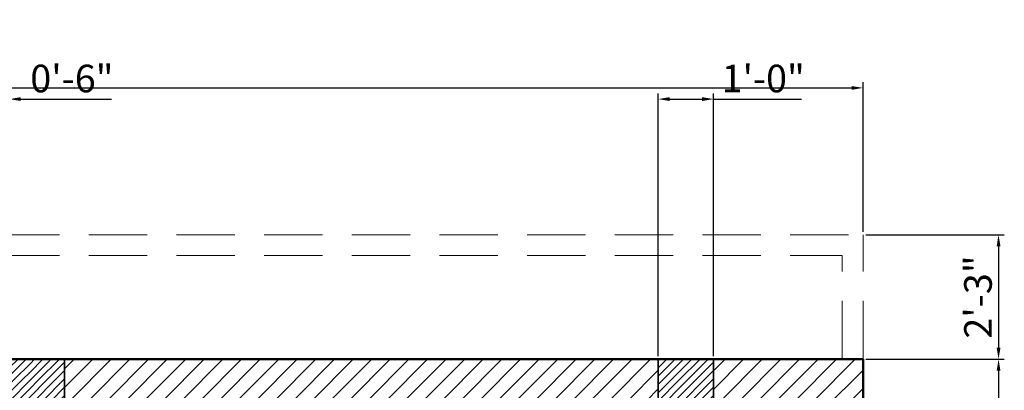
# Model space of a CAD drawing. Units: millimetres. Extents: x 225995 to 227247, y 225507 to 226008.
# Tile 23 of 23: x 227029 to 227243, y 225928 to 226008. Entities that reach past the tile are written whole.
import ezdxf

# ---------------------------------------------------------------- set-up
doc = ezdxf.new("R2010")
doc.units = ezdxf.units.MM
doc.linetypes.add('DASHED', pattern=[19.05, 12.7, -6.35])
for name, color, linetype, lineweight in [('A-ANNO-DIMS', 2, 'Continuous', 18), ('A-COLS', 40, 'Continuous', 35), ('A-WALL', 7, 'Continuous', 50), ('A-WALL-OVHD', 1, 'DASHED', 18), ('A-WALL-PATT', 8, 'Continuous', 13)]:
    doc.layers.add(name, color=color, linetype=linetype, lineweight=lineweight)
doc.styles.get("Standard").update_dxf_attribs({"font": 'arial.ttf'})
doc.dimstyles.new('ISO-25', dxfattribs={"dimtxt": 6, "dimasz": 2.5, "dimexe": 1.25, "dimexo": 0.625, "dimtad": 1, "dimdec": 0, "dimlunit": 3, "dimtxsty": 'Standard', "dimcen": 2.5, "dimadec": 0, "dimazin": 0, "dimtfac": 1, "dimtdec": 0, "dimtmove": 0, "dimatfit": 3, "dimfxl": 1, "dimarcsym": 0})
pattern_1 = [(45, (646.0463, 0.931), (-2.020557627, 2.020557627), [])]
pattern_2 = [(45, (787.0463, 234.931), (-0.898025612, 0.898025612), [])]
pattern_3 = [(45, (646.0463, 234.931), (-0.898025612, 0.898025612), [])]

# ---------------------------------------------------------------- blocks, each defined once
blk = doc.blocks.new('*D70')
at = {"layer": 'A-ANNO-DIMS', "color": 0, "lineweight": -2, "transparency": 16777216}
for p, q in [((226679.92, 225962.33), (226679.92, 225994.83)), ((226682.42, 225993.58), (227209.42, 225993.58)), ((227211.92, 225962.33), (227211.92, 225994.83))]:
    blk.add_line(p, q, dxfattribs=at)
at = {"layer": 'A-ANNO-DIMS', "color": 0, "transparency": 16777216}
for points in [[(226682.42, 225993.99), (226682.42, 225993.16), (226679.92, 225993.58)], [(227209.42, 225993.99), (227209.42, 225993.16), (227211.92, 225993.58)]]:
    blk.add_solid(points, dxfattribs=at)
at = {"layer": 'Defpoints', "color": 0, "transparency": 16777216}
for p in [(227211.92, 225993.58), (226679.92, 225961.7), (227211.92, 225961.7)]:
    blk.add_point(p, dxfattribs=at)
at = {"layer": 'A-ANNO-DIMS', "color": 0, "transparency": 16777216, "insert": (226945.92, 226000.2), "char_height": 12, "attachment_point": 5}
blk.add_mtext('44\'-4"', dxfattribs=at)
blk = doc.blocks.new('*D121')
at = {"layer": 'A-ANNO-DIMS', "color": 0, "lineweight": -2, "transparency": 16777216}
for p, q in [((227017.92, 225991.15), (227015.42, 225991.15)), ((227020.42, 225935.33), (227020.42, 225992.4)), ((227020.42, 225991.15), (227026.42, 225991.15)), ((227026.42, 225935.33), (227026.42, 225992.4)), ((227028.92, 225991.15), (227048.62, 225991.15))]:
    blk.add_line(p, q, dxfattribs=at)
at = {"layer": 'A-ANNO-DIMS', "color": 0, "transparency": 16777216}
for points in [[(227017.92, 225991.57), (227017.92, 225990.74), (227020.42, 225991.15)], [(227028.92, 225991.57), (227028.92, 225990.74), (227026.42, 225991.15)]]:
    blk.add_solid(points, dxfattribs=at)
at = {"layer": 'Defpoints', "color": 0, "transparency": 16777216}
for p in [(227026.42, 225991.15), (227020.42, 225934.7), (227026.42, 225934.7)]:
    blk.add_point(p, dxfattribs=at)
at = {"layer": 'A-ANNO-DIMS', "color": 0, "transparency": 16777216, "insert": (227040.02, 225994.84), "char_height": 6, "attachment_point": 5}
blk.add_mtext('0\'-6"', dxfattribs=at)
blk = doc.blocks.new('*D122')
at = {"layer": 'A-ANNO-DIMS', "color": 0, "lineweight": -2, "transparency": 16777216}
for p, q in [((227167.42, 225935.33), (227167.42, 225992.4)), ((227169.92, 225991.15), (227176.92, 225991.15)), ((227179.42, 225935.33), (227179.42, 225992.4)), ((227179.42, 225991.15), (227198.56, 225991.15))]:
    blk.add_line(p, q, dxfattribs=at)
at = {"layer": 'A-ANNO-DIMS', "color": 0, "transparency": 16777216}
for points in [[(227169.92, 225991.57), (227169.92, 225990.74), (227167.42, 225991.15)], [(227176.92, 225991.57), (227176.92, 225990.74), (227179.42, 225991.15)]]:
    blk.add_solid(points, dxfattribs=at)
at = {"layer": 'Defpoints', "color": 0, "transparency": 16777216}
for p in [(227179.42, 225991.15), (227167.42, 225934.7), (227179.42, 225934.7)]:
    blk.add_point(p, dxfattribs=at)
at = {"layer": 'A-ANNO-DIMS', "color": 0, "transparency": 16777216, "insert": (227190.24, 225994.84), "char_height": 6, "attachment_point": 5}
blk.add_mtext('1\'-0"', dxfattribs=at)
blk = doc.blocks.new('*D123')
at = {"layer": 'A-ANNO-DIMS', "color": 0, "lineweight": -2, "transparency": 16777216}
for p, q in [((227212.55, 225961.7), (227242.62, 225961.7)), ((227241.37, 225959.2), (227241.37, 225937.2)), ((227212.55, 225934.7), (227242.62, 225934.7))]:
    blk.add_line(p, q, dxfattribs=at)
at = {"layer": 'A-ANNO-DIMS', "color": 0, "transparency": 16777216}
for points in [[(227240.96, 225959.2), (227241.79, 225959.2), (227241.37, 225961.7)], [(227240.96, 225937.2), (227241.79, 225937.2), (227241.37, 225934.7)]]:
    blk.add_solid(points, dxfattribs=at)
at = {"layer": 'Defpoints', "color": 0, "transparency": 16777216}
for p in [(227211.92, 225961.7), (227211.92, 225934.7), (227241.37, 225934.7)]:
    blk.add_point(p, dxfattribs=at)
at = {"layer": 'A-ANNO-DIMS', "color": 0, "transparency": 16777216, "insert": (227237.68, 225948.2), "char_height": 6, "attachment_point": 5, "rotation": 90}
blk.add_mtext('2\'-3"', dxfattribs=at)
blk = doc.blocks.new('*D124')
at = {"layer": 'A-ANNO-DIMS', "color": 0, "lineweight": -2, "transparency": 16777216}
for p, q in [((227212.55, 225934.7), (227242.62, 225934.7)), ((227241.37, 225932.2), (227241.37, 225880.2)), ((227212.55, 225877.7), (227242.62, 225877.7))]:
    blk.add_line(p, q, dxfattribs=at)
at = {"layer": 'A-ANNO-DIMS', "color": 0, "transparency": 16777216}
for points in [[(227240.96, 225932.2), (227241.79, 225932.2), (227241.37, 225934.7)], [(227240.96, 225880.2), (227241.79, 225880.2), (227241.37, 225877.7)]]:
    blk.add_solid(points, dxfattribs=at)
at = {"layer": 'Defpoints', "color": 0, "transparency": 16777216}
for p in [(227211.92, 225934.7), (227211.92, 225877.7), (227241.37, 225877.7)]:
    blk.add_point(p, dxfattribs=at)
at = {"layer": 'A-ANNO-DIMS', "color": 0, "transparency": 16777216, "insert": (227237.68, 225906.2), "char_height": 6, "attachment_point": 5, "rotation": 90}
blk.add_mtext('4\'-9"', dxfattribs=at)

msp = doc.modelspace()

# ---------------------------------------------------------------- hatches: boundary and pattern name
at = {"layer": 'A-WALL-PATT'}
h = msp.add_hatch(dxfattribs=at)
h.set_pattern_fill('ANSI31', color=256, scale=0.4)
h.set_pattern_definition(pattern_3)
h.paths.add_polyline_path([(227030.92, 225934.7), (227026.42, 225934.7), (227026.42, 225930.2), (227030.92, 225930.2)])
h = msp.add_hatch(dxfattribs=at)
h.set_pattern_fill('ANSI31', color=256, scale=0.4)
h.set_pattern_definition(pattern_3)
h.paths.add_polyline_path([(227038.42, 225934.7), (227030.92, 225934.7), (227030.92, 225930.2), (227038.42, 225930.2)])
h = msp.add_hatch(dxfattribs=at)
h.set_pattern_fill('ANSI31', color=256, scale=0.9)
h.set_pattern_definition(pattern_1)
h.paths.add_polyline_path([(227167.42, 225934.7), (227038.42, 225934.7), (227038.42, 225925.7), (227167.42, 225925.7)])
h = msp.add_hatch(dxfattribs=at)
h.set_pattern_fill('ANSI31', color=256, scale=0.4)
h.set_pattern_definition(pattern_2)
h.paths.add_polyline_path([(227171.92, 225934.7), (227167.42, 225934.7), (227167.42, 225930.2), (227171.92, 225930.2)])
h = msp.add_hatch(dxfattribs=at)
h.set_pattern_fill('ANSI31', color=256, scale=0.4)
h.set_pattern_definition(pattern_2)
h.paths.add_polyline_path([(227179.42, 225934.7), (227171.92, 225934.7), (227171.92, 225930.2), (227179.42, 225930.2)])
h = msp.add_hatch(dxfattribs=at)
h.set_pattern_fill('ANSI31', color=256, scale=0.9)
h.set_pattern_definition(pattern_1)
h.paths.add_polyline_path([(227211.92, 225934.7), (227179.42, 225934.7), (227179.42, 225925.7), (227203.42, 225925.7), (227203.42, 225877.7), (227211.92, 225877.7)])
h = msp.add_hatch(dxfattribs=at)
h.set_pattern_fill('ANSI31', color=256, scale=0.4)
h.set_pattern_definition(pattern_3)
h.paths.add_polyline_path([(227030.92, 225930.2), (227026.42, 225930.2), (227026.42, 225925.7), (227030.92, 225925.7)])
h = msp.add_hatch(dxfattribs=at)
h.set_pattern_fill('ANSI31', color=256, scale=0.4)
h.set_pattern_definition(pattern_3)
h.paths.add_polyline_path([(227038.42, 225930.2), (227030.92, 225930.2), (227030.92, 225925.7), (227038.42, 225925.7)])
h = msp.add_hatch(dxfattribs=at)
h.set_pattern_fill('ANSI31', color=256, scale=0.4)
h.set_pattern_definition(pattern_2)
h.paths.add_polyline_path([(227171.92, 225930.2), (227167.42, 225930.2), (227167.42, 225925.7), (227171.92, 225925.7)])
h = msp.add_hatch(dxfattribs=at)
h.set_pattern_fill('ANSI31', color=256, scale=0.4)
h.set_pattern_definition(pattern_2)
h.paths.add_polyline_path([(227179.42, 225930.2), (227171.92, 225930.2), (227171.92, 225925.7), (227179.42, 225925.7)])

# ---------------------------------------------------------------- linework, layer by layer
at = {"layer": 'A-COLS'}
for points in [[(227026.42, 225925.7), (227026.42, 225934.7), (227038.42, 225934.7), (227038.42, 225925.7)], [(227167.42, 225925.7), (227167.42, 225934.7), (227179.42, 225934.7), (227179.42, 225925.7)]]:
    msp.add_lwpolyline(points, close=True, dxfattribs=at)
at = {"layer": 'A-WALL'}
for p, q in [((226757.92, 225934.7), (227211.92, 225934.7)), ((226757.92, 225934.7), (227211.92, 225934.7)), ((227211.92, 225934.7), (227211.92, 225571.7)), ((227211.92, 225934.7), (227211.92, 225571.7))]:
    msp.add_line(p, q, dxfattribs=at)
at = {"layer": 'A-WALL-OVHD'}
for p, q in [((226757.92, 225961.7), (227211.92, 225961.7)), ((227211.92, 225934.7), (227211.92, 225961.7)), ((226757.92, 225957.2), (227207.42, 225957.2)), ((227207.42, 225934.7), (227207.42, 225957.2))]:
    msp.add_line(p, q, dxfattribs=at)

# ---------------------------------------------------------------- dimensions: what is measured, and where the dimension line sits
at = {"layer": 'A-ANNO-DIMS'}
for base, p1, p2, override, picture, middle in [((227211.92, 225993.58), (226679.92, 225961.7), (227211.92, 225961.7), {"dimtxt": 12, "dimclrd": 0, "dimclre": 0, "dimclrt": 0}, '*D70', (226945.92, 226000.2)), ((227026.42, 225991.15), (227020.42, 225934.7), (227026.42, 225934.7), {"dimdec": 1, "dimlfac": 1, "dimrnd": 0, "dimzin": 1, "dimdsep": 46, "dimlunit": 4, "dimfrac": 2}, '*D121', (227040.02, 225994.84)), ((227179.42, 225991.15), (227167.42, 225934.7), (227179.42, 225934.7), {"dimdec": 1, "dimlfac": 1, "dimrnd": 0, "dimzin": 1, "dimdsep": 46, "dimlunit": 4, "dimfrac": 2}, '*D122', (227190.24, 225994.84))]:
    dim = msp.add_linear_dim(base=base, p1=p1, p2=p2, dimstyle='ISO-25', override=override, dxfattribs=at)
    dim.commit()
    dim.dimension.update_dxf_attribs({"geometry": picture, "text_midpoint": middle})
for base, p1, p2, picture, middle in [((227241.37, 225934.7), (227211.92, 225961.7), (227211.92, 225934.7), '*D123', (227237.68, 225948.2)), ((227241.37, 225877.7), (227211.92, 225934.7), (227211.92, 225877.7), '*D124', (227237.68, 225906.2))]:
    dim = msp.add_linear_dim(base=base, p1=p1, p2=p2, angle=90, dimstyle='ISO-25', override={"dimdec": 1, "dimlfac": 1, "dimrnd": 0, "dimzin": 1, "dimdsep": 46, "dimlunit": 4, "dimfrac": 2}, dxfattribs=at)
    dim.commit()
    dim.dimension.update_dxf_attribs({"geometry": picture, "text_midpoint": middle})

doc.saveas('drawing.dxf')
